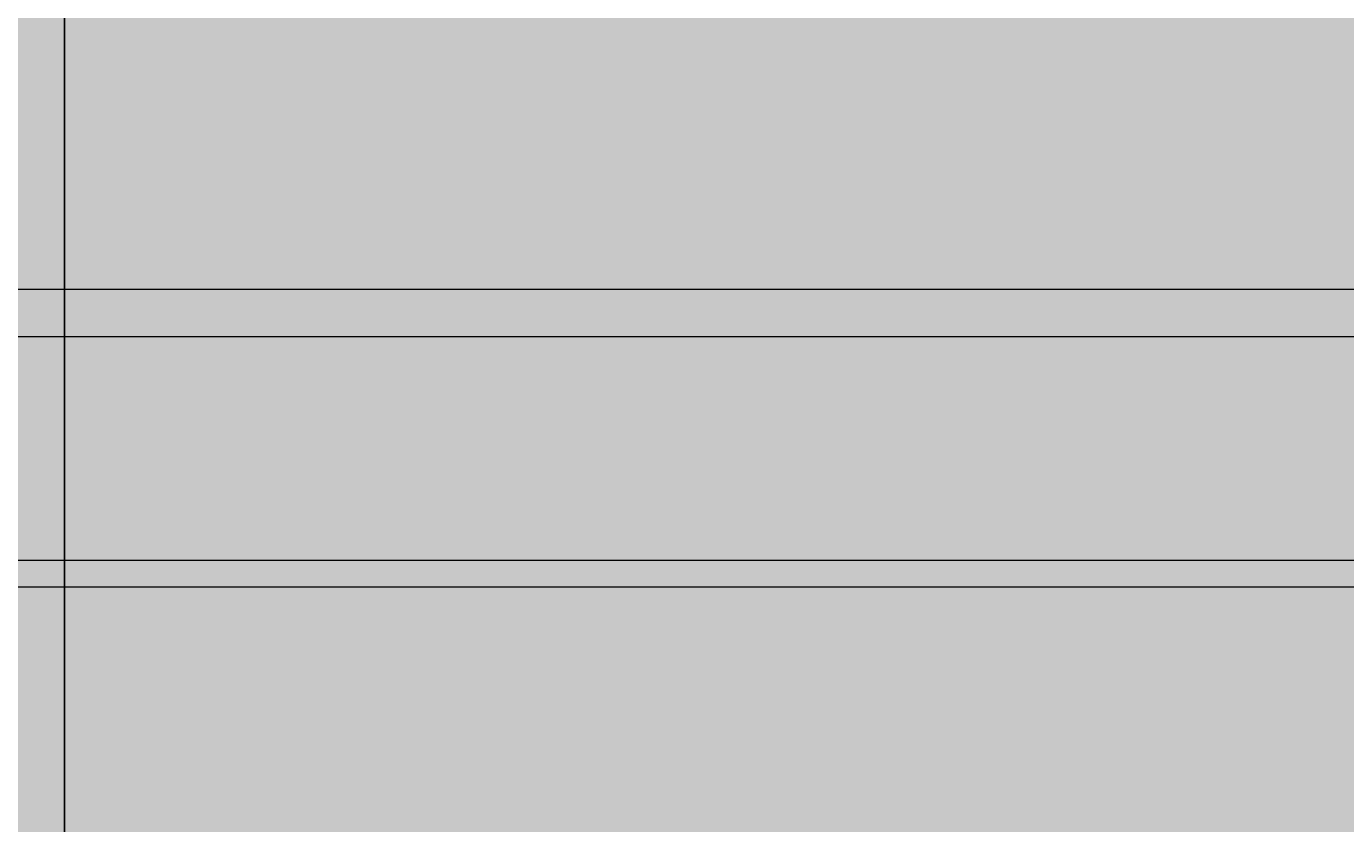
# Model space of a CAD drawing. Units: feet. Extents: x 2695 to 2912, y 795 to 1139.
# Tile 58 of 83: x 2843 to 2877, y 958 to 979. Entities that reach past the tile are written whole.
import ezdxf

# ---------------------------------------------------------------- set-up
doc = ezdxf.new("R2010")
doc.units = ezdxf.units.FT
for name, color, linetype, lineweight in [('A-ANNO-DIMS', 2, 'Continuous', 18), ('A-ELEV-PATT', 252, 'Continuous', 13), ('A-ELEV-RAIL', 8, 'Continuous', 18), ('A-GLAZ', 4, 'Continuous', 25)]:
    doc.layers.add(name, color=color, linetype=linetype, lineweight=lineweight)
doc.styles.get("Standard").update_dxf_attribs({"font": 'arial.ttf'})
doc.dimstyles.get("Standard").update_dxf_attribs({"dimtxt": 0.18, "dimasz": 0.18, "dimexe": 0.18, "dimexo": 0.0625, "dimgap": 0.09, "dimtad": 0, "dimtih": 1, "dimtoh": 1, "dimdec": 1, "dimzin": 0, "dimdsep": 46, "dimlunit": 3, "dimtxsty": 'Standard', "dimcen": 0.09, "dimadec": 0, "dimazin": 0, "dimtfac": 1, "dimtdec": 1, "dimtofl": 0, "dimtmove": 0, "dimatfit": 3, "dimfxl": 1, "dimtolj": 1, "dimtzin": 0, "dimarcsym": 0})

# ---------------------------------------------------------------- blocks, each defined once
blk = doc.blocks.new('*D17')
at = {"layer": 'A-ANNO-DIMS', "color": 0, "lineweight": -2, "transparency": 16777216}
for p, q in [((2843.637, 1020.824), (2911.424, 1020.824)), ((2911.244, 1020.644), (2911.244, 979.059)), ((2911.244, 937.111), (2911.244, 978.695)), ((2890.699, 936.931), (2911.424, 936.931))]:
    blk.add_line(p, q, dxfattribs=at)
at = {"layer": 'A-ANNO-DIMS', "color": 0, "transparency": 16777216}
for points in [[(2911.214, 1020.644), (2911.274, 1020.644), (2911.244, 1020.824)], [(2911.214, 937.111), (2911.274, 937.111), (2911.244, 936.931)]]:
    blk.add_solid(points, dxfattribs=at)
at = {"layer": 'Defpoints', "color": 0, "transparency": 16777216}
for p in [(2843.575, 1020.824), (2911.244, 1020.824), (2890.636, 936.931)]:
    blk.add_point(p, dxfattribs=at)
at = {"layer": 'A-ANNO-DIMS', "color": 0, "transparency": 16777216, "insert": (2911.244, 978.877), "char_height": 0.18, "attachment_point": 5}
blk.add_mtext('\\A1;83.9', dxfattribs=at)
blk = doc.blocks.new('*D50')
at = {"layer": 'A-ANNO-DIMS', "color": 0, "lineweight": -2, "transparency": 16777216}
for p, q in [((2810.041, 972.03), (2810.041, 1138.886)), ((2810.221, 1138.706), (2848.721, 1138.706)), ((2888.008, 1138.706), (2849.508, 1138.706)), ((2888.188, 972.03), (2888.188, 1138.886))]:
    blk.add_line(p, q, dxfattribs=at)
at = {"layer": 'A-ANNO-DIMS', "color": 0, "transparency": 16777216}
for points in [[(2810.221, 1138.736), (2810.221, 1138.676), (2810.041, 1138.706)], [(2888.008, 1138.736), (2888.008, 1138.676), (2888.188, 1138.706)]]:
    blk.add_solid(points, dxfattribs=at)
at = {"layer": 'Defpoints', "color": 0, "transparency": 16777216}
for p in [(2888.188, 1138.706), (2810.041, 971.967), (2888.188, 971.967)]:
    blk.add_point(p, dxfattribs=at)
at = {"layer": 'A-ANNO-DIMS', "color": 0, "transparency": 16777216, "insert": (2849.114, 1138.706), "char_height": 0.18, "attachment_point": 5}
blk.add_mtext('\\A1;78.15', dxfattribs=at)

msp = doc.modelspace()

# ---------------------------------------------------------------- hatches: boundary and pattern name
at = {"layer": 'A-ELEV-PATT'}
h = msp.add_hatch(color=256, dxfattribs=at)
h.set_gradient(color1=(147, 149, 152), color2=(147, 149, 152), tint=1)
h.paths.add_polyline_path([(2770.6361, 1118.4096), (2710.6361, 1118.4096), (2710.6361, 1062.9306), (2770.6361, 1062.9306)])
h.paths.add_polyline_path([(2890.6361, 1103.3378), (2770.6361, 1103.3378), (2770.6361, 1062.9306), (2890.6361, 1062.9306)])
h.paths.add_polyline_path([(2730.7081, 1048.1052), (2755.1125, 1048.1052), (2755.1125, 936.9306), (2770.6361, 936.9306), (2770.6361, 1050.3105), (2715.8852, 1050.3105), (2715.8852, 936.9306), (2730.7081, 936.9306)])
h.paths.add_polyline_path([(2890.6361, 1050.3105), (2770.6361, 1050.3105), (2770.6361, 971.9673), (2778.0341, 971.9673), (2778.0341, 1020.8235), (2843.575, 1020.8235), (2843.575, 971.9673), (2890.6361, 971.9673)])
h.paths.add_polyline_path([(2888.1882, 970.7156), (2843.575, 970.7156), (2843.575, 964.8267), (2888.1882, 964.8267)])
h.paths.add_polyline_path([(2888.1882, 964.1328), (2843.575, 964.1328), (2843.575, 956.614), (2888.1882, 956.614)])
h.paths.add_polyline_path([(2888.1882, 955.9202), (2843.575, 955.9202), (2843.575, 949.2892), (2888.1882, 949.2892)])
h.paths.add_polyline_path([(2888.1882, 948.5954), (2843.575, 948.5954), (2843.575, 941.3507), (2888.1882, 941.3507)])
h.paths.add_polyline_path([(2888.1882, 940.6569), (2843.575, 940.6569), (2843.575, 936.9306), (2888.1882, 936.9306)])
h.paths.add_polyline_path([(2890.6361, 970.7156), (2888.9368, 970.7156), (2888.9368, 964.8267), (2890.6361, 964.8267)])
h.paths.add_polyline_path([(2890.6361, 964.1328), (2888.9368, 964.1328), (2888.9368, 956.614), (2890.6361, 956.614)])
h.paths.add_polyline_path([(2890.6361, 955.9202), (2888.9368, 955.9202), (2888.9368, 949.2892), (2890.6361, 949.2892)])
h.paths.add_polyline_path([(2890.6361, 940.6569), (2888.9368, 940.6569), (2888.9368, 936.9306), (2890.6361, 936.9306)])
h.paths.add_polyline_path([(2890.6361, 948.5954), (2888.9368, 948.5954), (2888.9368, 941.3507), (2890.6361, 941.3507)])
h.paths.add_polyline_path([(2772.5216, 970.7156), (2770.6361, 970.7156), (2770.6361, 964.8267), (2772.5216, 964.8267)])
h.paths.add_polyline_path([(2772.5216, 964.1328), (2770.6361, 964.1328), (2770.6361, 956.614), (2772.5216, 956.614)])
h.paths.add_polyline_path([(2772.5216, 955.9202), (2770.6361, 955.9202), (2770.6361, 949.2892), (2772.5216, 949.2892)])
h.paths.add_polyline_path([(2772.5216, 948.5954), (2770.6361, 948.5954), (2770.6361, 941.3507), (2772.5216, 941.3507)])
h.paths.add_polyline_path([(2772.5216, 940.6569), (2770.6361, 940.6569), (2770.6361, 936.9306), (2772.5216, 936.9306)])
h.paths.add_polyline_path([(2778.0341, 940.6569), (2773.2702, 940.6569), (2773.2702, 936.9306), (2778.0341, 936.9306)])
h.paths.add_polyline_path([(2778.0341, 970.7156), (2773.2702, 970.7156), (2773.2702, 964.8267), (2778.0341, 964.8267)])
h.paths.add_polyline_path([(2778.0341, 964.1328), (2773.2702, 964.1328), (2773.2702, 956.614), (2778.0341, 956.614)])
h.paths.add_polyline_path([(2778.0341, 955.9202), (2773.2702, 955.9202), (2773.2702, 949.2892), (2778.0341, 949.2892)])
h.paths.add_polyline_path([(2778.0341, 948.5954), (2773.2702, 948.5954), (2773.2702, 941.3507), (2778.0341, 941.3507)])
h.paths.add_polyline_path([(2810.0407, 940.6569), (2780.0341, 940.6569), (2780.0341, 936.9306), (2810.0407, 936.9306)])
h.paths.add_polyline_path([(2890.6361, 924.3105), (2770.6361, 924.3105), (2770.6361, 810.9306), (2773.5029, 810.9306), (2773.5029, 905.5143), (2805.9398, 905.5143), (2838.3767, 905.5143), (2838.3767, 810.9306), (2890.6361, 810.9306)])
h = msp.add_hatch(color=256, dxfattribs=at)
h.set_gradient(color2=(0, 0, 0), tint=1)
h.paths.add_polyline_path([(2772.5216, 971.9673), (2770.6361, 971.9673), (2770.6361, 970.7156), (2772.5216, 970.7156)])
h.paths.add_polyline_path([(2773.2702, 971.9673), (2772.5216, 971.9673), (2772.5216, 970.7156), (2773.2702, 970.7156)])
h.paths.add_polyline_path([(2778.0341, 971.9673), (2773.2702, 971.9673), (2773.2702, 970.7156), (2778.0341, 970.7156)])
h.paths.add_polyline_path([(2780.0341, 971.9673), (2778.0341, 971.9673), (2778.0341, 970.7156), (2780.0341, 970.7156)])
h.paths.add_polyline_path([(2841.575, 971.9673), (2780.0341, 971.9673), (2780.0341, 970.7156), (2841.575, 970.7156)])
h.paths.add_polyline_path([(2843.575, 971.9673), (2841.575, 971.9673), (2841.575, 970.7156), (2843.575, 970.7156)])
h.paths.add_polyline_path([(2888.1882, 971.9673), (2843.575, 971.9673), (2843.575, 970.7156), (2888.1882, 970.7156)])
h.paths.add_polyline_path([(2888.9368, 971.9673), (2888.1882, 971.9673), (2888.1882, 970.7156), (2888.9368, 970.7156)], flags=17)
h.paths.add_polyline_path([(2890.6361, 971.9673), (2888.9368, 971.9673), (2888.9368, 970.7156), (2890.6361, 970.7156)])
h.paths.add_polyline_path([(2888.9368, 971.9673), (2888.1882, 971.9673), (2888.1882, 964.8267), (2888.9368, 964.8267)])
h.paths.add_polyline_path([(2888.9368, 964.8267), (2888.1882, 964.8267), (2888.1882, 964.1328), (2888.9368, 964.1328)])
h.paths.add_polyline_path([(2890.6361, 964.8267), (2888.9368, 964.8267), (2888.9368, 964.1328), (2890.6361, 964.1328)])
h.paths.add_polyline_path([(2888.1882, 964.8267), (2770.6361, 964.8267), (2770.6361, 964.1328), (2888.1882, 964.1328)])
h.paths.add_polyline_path([(2888.9368, 964.1328), (2888.1882, 964.1328), (2888.1882, 936.9306), (2888.9368, 936.9306)])
h.paths.add_polyline_path([(2890.6361, 956.614), (2888.9368, 956.614), (2888.9368, 955.9202), (2890.6361, 955.9202)])
h.paths.add_polyline_path([(2888.1882, 956.614), (2770.6361, 956.614), (2770.6361, 955.9202), (2888.1882, 955.9202)])
h.paths.add_polyline_path([(2890.6361, 949.2892), (2888.9368, 949.2892), (2888.9368, 948.5954), (2890.6361, 948.5954)])
h.paths.add_polyline_path([(2888.1882, 949.2892), (2770.6361, 949.2892), (2770.6361, 948.5954), (2888.1882, 948.5954)])
h.paths.add_polyline_path([(2890.6361, 941.3507), (2888.9368, 941.3507), (2888.9368, 940.6569), (2890.6361, 940.6569)])
h.paths.add_polyline_path([(2888.1882, 941.3507), (2770.6361, 941.3507), (2770.6361, 940.6569), (2888.1882, 940.6569)])
h.paths.add_polyline_path([(2773.2702, 970.7156), (2772.5216, 970.7156), (2772.5216, 964.8267), (2773.2702, 964.8267)])
h.paths.add_polyline_path([(2773.2702, 964.1328), (2772.5216, 964.1328), (2772.5216, 956.614), (2773.2702, 956.614)])
h.paths.add_polyline_path([(2773.2702, 955.9202), (2772.5216, 955.9202), (2772.5216, 936.9306), (2773.2702, 936.9306)])
h.paths.add_polyline_path([(2810.7893, 970.7156), (2810.0407, 970.7156), (2810.0407, 964.8267), (2810.7893, 964.8267)], flags=17)
h.paths.add_polyline_path([(2810.7893, 964.1328), (2810.0407, 964.1328), (2810.0407, 956.614), (2810.7893, 956.614)], flags=17)
h.paths.add_polyline_path([(2810.7893, 955.9202), (2810.0407, 955.9202), (2810.0407, 949.2892), (2810.7893, 949.2892)], flags=17)
h.paths.add_polyline_path([(2810.7893, 971.9673), (2810.0407, 971.9673), (2810.0407, 941.3507), (2810.7893, 941.3507)])
h.paths.add_polyline_path([(2810.7893, 940.6569), (2810.0407, 940.6569), (2810.0407, 936.9306), (2810.7893, 936.9306)])
h.paths.add_polyline_path([(2780.0341, 1018.8235), (2841.575, 1018.8235), (2841.575, 971.9673), (2843.575, 971.9673), (2843.575, 1020.8235), (2778.0341, 1020.8235), (2778.0341, 971.9673), (2780.0341, 971.9673)])
h.paths.add_polyline_path([(2780.0341, 970.7156), (2778.0341, 970.7156), (2778.0341, 964.8267), (2780.0341, 964.8267)])
h.paths.add_polyline_path([(2780.0341, 964.1328), (2778.0341, 964.1328), (2778.0341, 956.614), (2780.0341, 956.614)])
h.paths.add_polyline_path([(2780.0341, 955.9202), (2778.0341, 955.9202), (2778.0341, 949.2892), (2780.0341, 949.2892)])
h.paths.add_polyline_path([(2780.0341, 948.5954), (2778.0341, 948.5954), (2778.0341, 941.3507), (2780.0341, 941.3507)])
h.paths.add_polyline_path([(2780.0341, 940.6569), (2778.0341, 940.6569), (2778.0341, 936.9306), (2780.0341, 936.9306)])
h.paths.add_polyline_path([(2843.575, 940.6569), (2841.575, 940.6569), (2841.575, 936.9306), (2843.575, 936.9306)])
h.paths.add_polyline_path([(2843.575, 948.5954), (2841.575, 948.5954), (2841.575, 941.3507), (2843.575, 941.3507)])
h.paths.add_polyline_path([(2843.575, 970.7156), (2841.575, 970.7156), (2841.575, 964.8267), (2843.575, 964.8267)])
h.paths.add_polyline_path([(2843.575, 964.1328), (2841.575, 964.1328), (2841.575, 956.614), (2843.575, 956.614)])
h.paths.add_polyline_path([(2843.575, 955.9202), (2841.575, 955.9202), (2841.575, 949.2892), (2843.575, 949.2892)])
h.paths.add_polyline_path([(2805.0538, 874.1057), (2803.9681, 874.1057), (2803.9681, 846.2857), (2805.0538, 846.2857)])
h.paths.add_polyline_path([(2758.1515, 902.577), (2724.1893, 902.577), (2724.1893, 874.8571), (2758.1515, 874.8571)])
h.paths.add_polyline_path([(2726.1893, 900.577), (2756.1515, 900.577), (2756.1515, 876.8571), (2726.1893, 876.8571)], flags=16)
h.paths.add_polyline_path([(2740.7302, 900.577), (2741.6105, 900.577), (2741.6105, 876.8571), (2740.7302, 876.8571)], flags=0)

# ---------------------------------------------------------------- linework, layer by layer
at = {"layer": 'A-ELEV-RAIL'}
msp.add_line((2770.6361, 971.9673), (2890.6361, 971.9673), dxfattribs=at)
msp.add_lwpolyline([(2770.6361, 970.7156), (2890.6361, 970.7156)], dxfattribs=at)
msp.add_lwpolyline([(2770.6361, 964.1328), (2890.6361, 964.1328), (2890.6361, 964.8267), (2770.6361, 964.8267)], close=True, dxfattribs=at)
at = {"layer": 'A-GLAZ'}
msp.add_lwpolyline([(2778.0341, 936.9306), (2778.0341, 1020.8235), (2843.575, 1020.8235), (2843.575, 936.9306)], dxfattribs=at)

# ---------------------------------------------------------------- dimensions: what is measured, and where the dimension line sits
at = {"layer": 'A-ANNO-DIMS'}
dim = msp.add_linear_dim(base=(2888.1882, 1138.7056), p1=(2810.0407, 971.9673), p2=(2888.1882, 971.9673), dimstyle='Standard', override={"dimdec": 2, "dimlfac": 1, "dimrnd": 0, "dimzin": 0, "dimdsep": 46, "dimlunit": 2}, dxfattribs=at)
dim.commit()
dim.dimension.update_dxf_attribs({"geometry": '*D50', "text_midpoint": (2849.1144, 1138.7056)})
dim = msp.add_linear_dim(base=(2911.2444, 1020.8235), p1=(2890.6361, 936.9306), p2=(2843.575, 1020.8235), angle=90, dimstyle='Standard', override={"dimdec": 1, "dimlfac": 1, "dimrnd": 0, "dimzin": 0, "dimdsep": 46, "dimlunit": 2}, dxfattribs=at)
dim.commit()
dim.dimension.update_dxf_attribs({"geometry": '*D17', "text_midpoint": (2911.2444, 978.877)})

doc.saveas('drawing.dxf')
